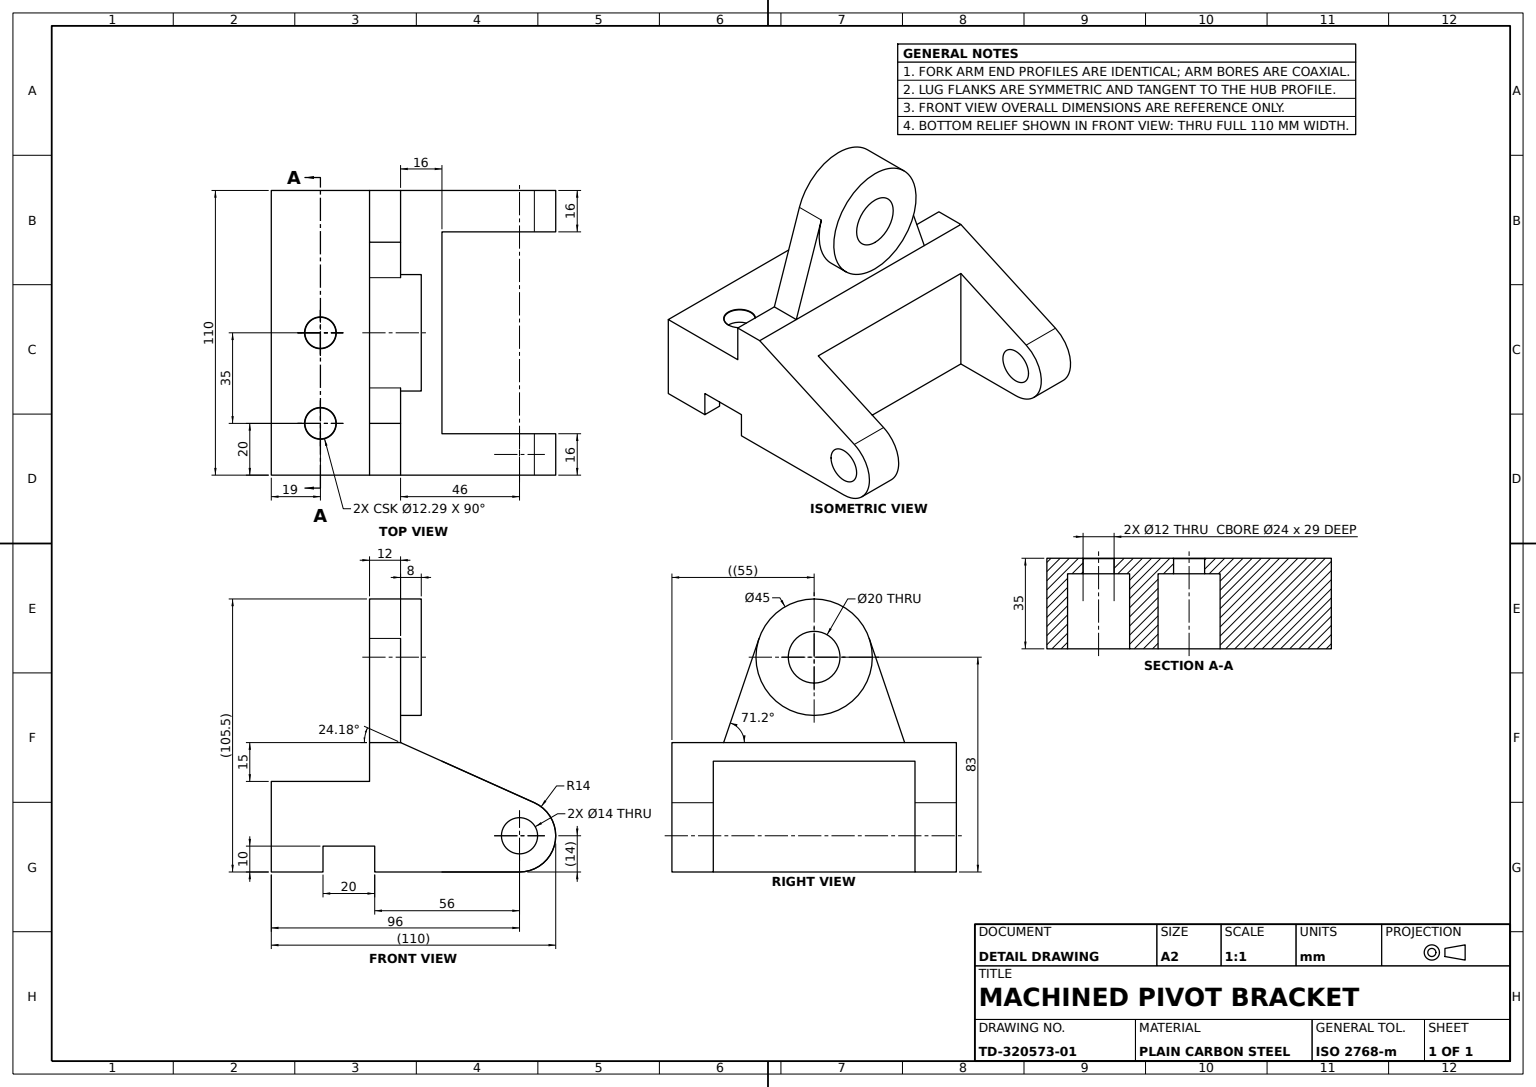
from build123d import *

# Parameters (mm, degrees)
BASE_BLOCK_PROFILE_SKETCH_W       = 96
BASE_BLOCK_PROFILE_SKETCH_H       = 35
BASE_BLOCK_DEPTH                  = 55
BASE_STEP_RECESS_DEPTH            = 81.956778592
BASE_STEP_RECESS_DEPTH_BACK       = 35
BASE_GROOVE_20X20_SKETCH_W        = 20
BASE_GROOVE_20X20_SKETCH_H        = 10
BASE_GROOVE_20X20_DEPTH           = 110
UPRIGHT_PAD_SKETCH_W              = 12
UPRIGHT_PAD_SKETCH_H              = 110
UPRIGHT_PAD_DEPTH                 = 15
LUG_PLATE_DEPTH                   = 12
LUG_START                         = 8
LUG_HUB_SKETCH_R                  = 22.5
LUG_HUB_DEPTH                     = 8
LUG_BORE_20_SKETCH_R              = 10
LUG_BORE_20_DEPTH                 = 20
SIDE_ARM_A_DEPTH                  = 16
SIDE_START                        = -16
SIDE_ARM_B_DEPTH                  = 16
ARM_B_EYE_HOLE_14_SKETCH_R        = 7
ARM_B_EYE_HOLE_14_DEPTH           = 16
ARM_START                         = -16
ARM_A_EYE_HOLE_14_SKETCH_R        = 7
ARM_A_EYE_HOLE_14_DEPTH           = 16
CROSS_WEB_SKETCH_W                = 16
CROSS_WEB_SKETCH_H                = 78
CROSS_WEB_DEPTH                   = 50
TRIANGULAR_RELIEF_CUT_REACH       = 156.306
COUNTERBORED_BOLT_HOLE_AT_2_COUNT = 2
COUNTERBORED_BOLT_HOLE_AT_2_PITCH = 35


with BuildPart() as part:
    # Base Block Profile Sketch → Base Block (new, symmetric)
    with BuildSketch(Plane.XY):
        with Locations((0, 17.5)):
            Rectangle(BASE_BLOCK_PROFILE_SKETCH_W, BASE_BLOCK_PROFILE_SKETCH_H)
    extrude(amount=BASE_BLOCK_DEPTH, both=True)

    # Base Step Recess Sketch → Base Step Recess (cut, two sides: drawn at the far end of the back side and taken through both)
    with BuildSketch(Plane(origin=(0, 35, 0), x_dir=(1, 0, 0), z_dir=(0, 1, 0)).offset(-BASE_STEP_RECESS_DEPTH_BACK)):
        Polygon((48, 55), (47.003525264, 55), (2, 55), (2, -55), (48, -55), align=None)
    extrude(amount=BASE_STEP_RECESS_DEPTH + BASE_STEP_RECESS_DEPTH_BACK, mode=Mode.SUBTRACT)

    # Base Groove 20x20 Sketch → Base Groove 20x20 (cut)
    with BuildSketch(Plane.XY.offset(55)):
        with Locations((-18, 5)):
            Rectangle(BASE_GROOVE_20X20_SKETCH_W, BASE_GROOVE_20X20_SKETCH_H)
    extrude(amount=-BASE_GROOVE_20X20_DEPTH, mode=Mode.SUBTRACT)

    # Upright Pad Sketch → Upright Pad (add)
    with BuildSketch(Plane(origin=(0, 35, 0), x_dir=(1, 0, 0), z_dir=(0, 1, 0))):
        with Locations((-4, 0)):
            Rectangle(UPRIGHT_PAD_SKETCH_W, UPRIGHT_PAD_SKETCH_H)
    extrude(amount=UPRIGHT_PAD_DEPTH)

    # Lug Plate Sketch → Lug Plate (add)
    with BuildSketch(Plane(origin=(2, 0, 0), x_dir=(0, 0, -1), z_dir=(1, 0, 0))):
        with BuildLine():
            Line((-35, 50), (-21.299956881, 90.249954267))
            ThreePointArc((-21.299956881, 90.249954267), (0, 105.5), (21.299956881, 90.249954267))
            Line((21.299956881, 90.249954267), (35, 50))
            Line((35, 50), (0, 50))
            Line((0, 50), (-35, 50))
        make_face()
    extrude(amount=-LUG_PLATE_DEPTH)

    # Lug Hub Sketch → Lug Hub (add)
    with BuildSketch(Plane(origin=(2, 0, 0), x_dir=(0, 0, -1), z_dir=(1, 0, 0)).offset(LUG_START)):
        with Locations(Location((0, 83, 0), (0, 0, 90))):
            Circle(LUG_HUB_SKETCH_R)
    extrude(amount=-LUG_HUB_DEPTH)

    # Lug Bore Ø20 Sketch → Lug Bore Ø20 (cut)
    with BuildSketch(Plane(origin=(10, 0, 0), x_dir=(0, 0, -1), z_dir=(1, 0, 0))):
        with Locations(Location((0, 83, 0), (0, 0, 90))):
            Circle(LUG_BORE_20_SKETCH_R)
    extrude(amount=-LUG_BORE_20_DEPTH, mode=Mode.SUBTRACT)

    # Side Arm A Sketch → Side Arm A (add)
    with BuildSketch(Plane(origin=(0, 0, -55), x_dir=(-1, 0, 0), z_dir=(0, 0, -1))):
        with BuildLine():
            Line((8, 0), (-48, 0))
            ThreePointArc((-48, 0), (-61.689486066, 11.067770261), (-53.734388308, 26.771718394))
            Line((-53.734388308, 26.771718394), (-2, 50))
            Line((-2, 50), (10, 50))
            Line((10, 50), (10, 35))
            Line((10, 35), (10, 10))
            Line((10, 10), (8, 10))
            Line((8, 10), (8, 0))
        make_face()
    extrude(amount=-SIDE_ARM_A_DEPTH)

    # Side Arm B Sketch → Side Arm B (add)
    with BuildSketch(Plane.XY.offset(55).offset(SIDE_START)):
        with BuildLine():
            Line((-8, 0), (48, 0))
            ThreePointArc((48, 0), (61.689486066, 11.067770261), (53.734388308, 26.771718394))
            Line((53.734388308, 26.771718394), (2, 50))
            Line((2, 50), (-10, 50))
            Line((-10, 50), (-10, 35))
            Line((-10, 35), (-13.136025353, 35))
            Line((-13.136025353, 35), (-13.136025353, 10))
            Line((-13.136025353, 10), (-8, 10))
            Line((-8, 10), (-8, 0))
        make_face()
    extrude(amount=SIDE_ARM_B_DEPTH)

    # Arm B Eye Hole Ø14 Sketch → Arm B Eye Hole Ø14 (cut)
    with BuildSketch(Plane.XY.offset(55)):
        with Locations((48, 14)):
            Circle(ARM_B_EYE_HOLE_14_SKETCH_R)
    extrude(amount=-ARM_B_EYE_HOLE_14_DEPTH, mode=Mode.SUBTRACT)

    # Arm A Eye Hole Ø14 Sketch → Arm A Eye Hole Ø14 (cut)
    with BuildSketch(Plane(origin=(0, 0, -55), x_dir=(-1, 0, 0), z_dir=(0, 0, -1)).offset(ARM_START)):
        with Locations(Location((-48, 14, 0), (0, 0, 180))):
            Circle(ARM_A_EYE_HOLE_14_SKETCH_R)
    extrude(amount=ARM_A_EYE_HOLE_14_DEPTH, mode=Mode.SUBTRACT)

    # Cross Web Sketch → Cross Web (add)
    with BuildSketch(Plane(origin=(0, 50, 0), x_dir=(1, 0, 0), z_dir=(0, 1, 0))):
        with Locations((10, 0)):
            Rectangle(CROSS_WEB_SKETCH_W, CROSS_WEB_SKETCH_H)
    extrude(amount=-CROSS_WEB_DEPTH)

    # Triangular Relief Sketch → Triangular Relief Cut (cut, up to next)
    with BuildSketch(Plane.XY.offset(39), mode=Mode.PRIVATE) as triangular_relief_cut_sk1:
        Polygon((2, 50), (18, 42.816141877), (18, 50), align=None)
    triangular_relief_cut_tool1 = extrude(triangular_relief_cut_sk1.sketch, amount=-TRIANGULAR_RELIEF_CUT_REACH, mode=Mode.PRIVATE) & part.part
    add(triangular_relief_cut_tool1.solids().sort_by_distance((12.666667, 47.605381, 39))[0], mode=Mode.SUBTRACT)

    # Sketch42 → Counterbored Bolt Hole (revolve, cut)
    with BuildSketch(Plane(origin=(-29, 35, 35), x_dir=(0, 0, 1), z_dir=(1, 0, 0))):
        Polygon((0, 0), (0, 35), (12, 35), (12, 6), (6, 6), (6, 0.145), (6.145, 0), align=None)
    counterbored_bolt_hole = revolve(axis=Axis((-29, 41.35, 35), (0, -1, 0)), mode=Mode.SUBTRACT)

    # Counterbored Bolt Hole at 2: Counterbored Bolt Hole ×2
    with Locations(*[(0, 0, -i * COUNTERBORED_BOLT_HOLE_AT_2_PITCH) for i in range(1, COUNTERBORED_BOLT_HOLE_AT_2_COUNT)]):
        add(counterbored_bolt_hole, mode=Mode.SUBTRACT)


solid = part.part
